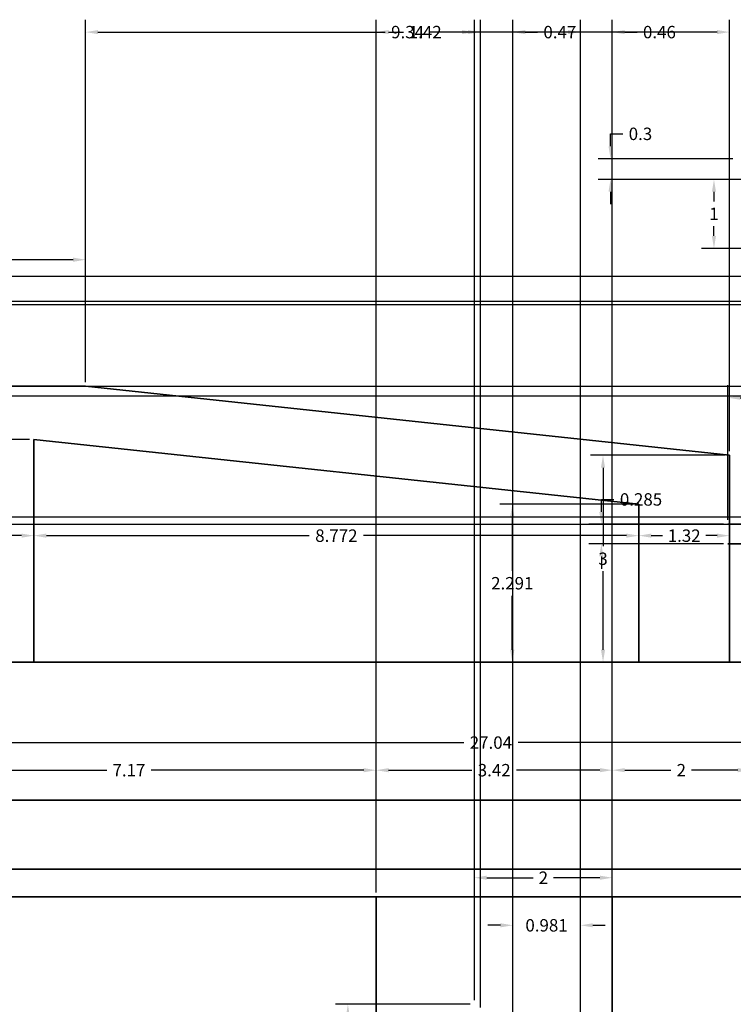
# Model space of a CAD drawing. Units: millimetres. Extents: x 2473 to 2512.3, y 2191.3 to 2230.4.
# Tile 5 of 8: x 2483.3 to 2493.7, y 2216.1 to 2230.4. Entities that reach past the tile are written whole.
import ezdxf

# ---------------------------------------------------------------- set-up
doc = ezdxf.new("R2010")
doc.units = ezdxf.units.MM
doc.layers.add('A-ANNO-DIMS', color=2, linetype='Continuous', lineweight=18)
doc.layers.add('A-ELEV', color=7, linetype='Continuous', lineweight=35)
doc.styles.get("Standard").update_dxf_attribs({"font": 'arial.ttf'})
doc.dimstyles.get("Standard").update_dxf_attribs({"dimtxt": 0.18, "dimasz": 0.18, "dimexe": 0.18, "dimexo": 0.0625, "dimgap": 0.09, "dimtad": 0, "dimtih": 1, "dimtoh": 1, "dimdec": 4, "dimzin": 0, "dimdsep": 46, "dimtxsty": 'Standard', "dimcen": 0.09, "dimadec": 0, "dimazin": 0, "dimtfac": 1, "dimtdec": 4, "dimtofl": 0, "dimtmove": 0, "dimatfit": 3, "dimfxl": 1, "dimtolj": 1, "dimtzin": 0, "dimarcsym": 0})

# ---------------------------------------------------------------- blocks, each defined once
blk = doc.blocks.new('*D18')
at = {"layer": 'A-ANNO-DIMS', "color": 0, "lineweight": -2, "transparency": 16777216}
for p, q in [((2476.623, 2218.117), (2476.623, 2220.07)), ((2503.664, 2218.117), (2503.664, 2220.07)), ((2476.803, 2219.89), (2489.749, 2219.89)), ((2503.484, 2219.89), (2490.538, 2219.89))]:
    blk.add_line(p, q, dxfattribs=at)
at = {"layer": 'A-ANNO-DIMS', "color": 0, "transparency": 16777216}
for points in [[(2476.803, 2219.92), (2476.803, 2219.86), (2476.623, 2219.89)], [(2503.484, 2219.92), (2503.484, 2219.86), (2503.664, 2219.89)]]:
    blk.add_solid(points, dxfattribs=at)
at = {"layer": 'Defpoints', "color": 0, "transparency": 16777216}
for p in [(2503.664, 2219.89), (2476.623, 2218.055), (2503.664, 2218.055)]:
    blk.add_point(p, dxfattribs=at)
at = {"layer": 'A-ANNO-DIMS', "color": 0, "transparency": 16777216, "insert": (2490.143, 2219.89), "char_height": 0.18, "attachment_point": 5}
blk.add_mtext('\\A1;27.04', dxfattribs=at)
blk = doc.blocks.new('*D48')
at = {"layer": 'A-ANNO-DIMS', "color": 0, "lineweight": -2, "transparency": 16777216}
for p, q in [((2481.31, 2217.717), (2481.31, 2219.67)), ((2488.479, 2217.717), (2488.479, 2219.67)), ((2481.49, 2219.49), (2484.571, 2219.49)), ((2488.299, 2219.49), (2485.217, 2219.49))]:
    blk.add_line(p, q, dxfattribs=at)
at = {"layer": 'A-ANNO-DIMS', "color": 0, "transparency": 16777216}
for points in [[(2481.49, 2219.52), (2481.49, 2219.46), (2481.31, 2219.49)], [(2488.299, 2219.52), (2488.299, 2219.46), (2488.479, 2219.49)]]:
    blk.add_solid(points, dxfattribs=at)
at = {"layer": 'Defpoints', "color": 0, "transparency": 16777216}
for p in [(2488.479, 2219.49), (2481.31, 2217.655), (2488.479, 2217.655)]:
    blk.add_point(p, dxfattribs=at)
at = {"layer": 'A-ANNO-DIMS', "color": 0, "transparency": 16777216, "insert": (2484.894, 2219.49), "char_height": 0.18, "attachment_point": 5}
blk.add_mtext('\\A1;7.17', dxfattribs=at)
blk = doc.blocks.new('*D49')
at = {"layer": 'A-ANNO-DIMS', "color": 0, "lineweight": -2, "transparency": 16777216}
for p, q in [((2488.479, 2217.717), (2488.479, 2219.67)), ((2491.904, 2217.717), (2491.904, 2219.67)), ((2488.659, 2219.49), (2489.868, 2219.49)), ((2491.724, 2219.49), (2490.514, 2219.49))]:
    blk.add_line(p, q, dxfattribs=at)
at = {"layer": 'A-ANNO-DIMS', "color": 0, "transparency": 16777216}
for points in [[(2488.659, 2219.52), (2488.659, 2219.46), (2488.479, 2219.49)], [(2491.724, 2219.52), (2491.724, 2219.46), (2491.904, 2219.49)]]:
    blk.add_solid(points, dxfattribs=at)
at = {"layer": 'Defpoints', "color": 0, "transparency": 16777216}
for p in [(2491.904, 2219.49), (2488.479, 2217.655), (2491.904, 2217.655)]:
    blk.add_point(p, dxfattribs=at)
at = {"layer": 'A-ANNO-DIMS', "color": 0, "transparency": 16777216, "insert": (2490.191, 2219.49), "char_height": 0.18, "attachment_point": 5}
blk.add_mtext('\\A1;3.42', dxfattribs=at)
blk = doc.blocks.new('*D50')
at = {"layer": 'A-ANNO-DIMS', "color": 0, "lineweight": -2, "transparency": 16777216}
for p, q in [((2491.904, 2217.717), (2491.904, 2219.67)), ((2493.904, 2217.717), (2493.904, 2219.67)), ((2492.084, 2219.49), (2492.754, 2219.49)), ((2493.724, 2219.49), (2493.053, 2219.49))]:
    blk.add_line(p, q, dxfattribs=at)
at = {"layer": 'A-ANNO-DIMS', "color": 0, "transparency": 16777216}
for points in [[(2492.084, 2219.52), (2492.084, 2219.46), (2491.904, 2219.49)], [(2493.724, 2219.52), (2493.724, 2219.46), (2493.904, 2219.49)]]:
    blk.add_solid(points, dxfattribs=at)
at = {"layer": 'Defpoints', "color": 0, "transparency": 16777216}
for p in [(2493.904, 2219.49), (2491.904, 2217.655), (2493.904, 2217.655)]:
    blk.add_point(p, dxfattribs=at)
at = {"layer": 'A-ANNO-DIMS', "color": 0, "transparency": 16777216, "insert": (2492.904, 2219.49), "char_height": 0.18, "attachment_point": 5}
blk.add_mtext('\\A1;2', dxfattribs=at)
blk = doc.blocks.new('*D56')
at = {"layer": 'A-ANNO-DIMS', "color": 0, "lineweight": -2, "transparency": 16777216}
for p, q in [((2488.479, 2217.717), (2488.479, 2230.37)), ((2489.904, 2216.158), (2489.904, 2230.37)), ((2488.659, 2230.19), (2488.877, 2230.19)), ((2489.724, 2230.19), (2489.506, 2230.19))]:
    blk.add_line(p, q, dxfattribs=at)
at = {"layer": 'A-ANNO-DIMS', "color": 0, "transparency": 16777216}
for points in [[(2488.659, 2230.22), (2488.659, 2230.16), (2488.479, 2230.19)], [(2489.724, 2230.22), (2489.724, 2230.16), (2489.904, 2230.19)]]:
    blk.add_solid(points, dxfattribs=at)
at = {"layer": 'Defpoints', "color": 0, "transparency": 16777216}
for p in [(2489.904, 2230.19), (2488.479, 2217.655), (2489.904, 2216.096)]:
    blk.add_point(p, dxfattribs=at)
at = {"layer": 'A-ANNO-DIMS', "color": 0, "transparency": 16777216, "insert": (2489.191, 2230.19), "char_height": 0.18, "attachment_point": 5}
blk.add_mtext('\\A1;1.42', dxfattribs=at)
blk = doc.blocks.new('*D57')
at = {"layer": 'A-ANNO-DIMS', "color": 0, "lineweight": -2, "transparency": 16777216}
for p, q in [((2489.904, 2216.158), (2489.904, 2218.111)), ((2491.904, 2216.158), (2491.904, 2218.111)), ((2490.084, 2217.931), (2490.754, 2217.931)), ((2491.724, 2217.931), (2491.053, 2217.931))]:
    blk.add_line(p, q, dxfattribs=at)
at = {"layer": 'A-ANNO-DIMS', "color": 0, "transparency": 16777216}
for points in [[(2490.084, 2217.961), (2490.084, 2217.901), (2489.904, 2217.931)], [(2491.724, 2217.961), (2491.724, 2217.901), (2491.904, 2217.931)]]:
    blk.add_solid(points, dxfattribs=at)
at = {"layer": 'Defpoints', "color": 0, "transparency": 16777216}
for p in [(2491.904, 2217.931), (2489.904, 2216.096), (2491.904, 2216.096)]:
    blk.add_point(p, dxfattribs=at)
at = {"layer": 'A-ANNO-DIMS', "color": 0, "transparency": 16777216, "insert": (2490.904, 2217.931), "char_height": 0.18, "attachment_point": 5}
blk.add_mtext('\\A1;2', dxfattribs=at)
blk = doc.blocks.new('*D58')
at = {"layer": 'A-ANNO-DIMS', "color": 0, "lineweight": -2, "transparency": 16777216}
for p, q in [((2490.46, 2215.468), (2490.46, 2217.421)), ((2491.441, 2215.468), (2491.441, 2217.421)), ((2490.28, 2217.241), (2490.1, 2217.241)), ((2491.621, 2217.241), (2491.801, 2217.241))]:
    blk.add_line(p, q, dxfattribs=at)
at = {"layer": 'A-ANNO-DIMS', "color": 0, "transparency": 16777216}
for points in [[(2490.28, 2217.271), (2490.28, 2217.211), (2490.46, 2217.241)], [(2491.621, 2217.271), (2491.621, 2217.211), (2491.441, 2217.241)]]:
    blk.add_solid(points, dxfattribs=at)
at = {"layer": 'Defpoints', "color": 0, "transparency": 16777216}
for p in [(2491.441, 2217.241), (2490.46, 2215.406), (2491.441, 2215.406)]:
    blk.add_point(p, dxfattribs=at)
at = {"layer": 'A-ANNO-DIMS', "color": 0, "transparency": 16777216, "insert": (2490.95, 2217.241), "char_height": 0.18, "attachment_point": 5}
blk.add_mtext('\\A1;0.981', dxfattribs=at)
blk = doc.blocks.new('*D59')
at = {"layer": 'A-ANNO-DIMS', "color": 0, "lineweight": -2, "transparency": 16777216}
for p, q in [((2489.841, 2216.096), (2487.889, 2216.096)), ((2488.069, 2215.916), (2488.069, 2212.957)), ((2488.069, 2209.635), (2488.069, 2212.593)), ((2489.841, 2209.455), (2487.889, 2209.455))]:
    blk.add_line(p, q, dxfattribs=at)
at = {"layer": 'A-ANNO-DIMS', "color": 0, "transparency": 16777216}
for points in [[(2488.039, 2215.916), (2488.099, 2215.916), (2488.069, 2216.096)], [(2488.039, 2209.635), (2488.099, 2209.635), (2488.069, 2209.455)]]:
    blk.add_solid(points, dxfattribs=at)
at = {"layer": 'Defpoints', "color": 0, "transparency": 16777216}
for p in [(2488.069, 2216.096), (2489.904, 2216.096), (2489.904, 2209.455)]:
    blk.add_point(p, dxfattribs=at)
at = {"layer": 'A-ANNO-DIMS', "color": 0, "transparency": 16777216, "insert": (2488.069, 2212.775), "char_height": 0.18, "attachment_point": 5}
blk.add_mtext('\\A1;6.641', dxfattribs=at)
blk = doc.blocks.new('*D72')
at = {"layer": 'A-ANNO-DIMS', "color": 0, "lineweight": -2, "transparency": 16777216}
for p, q in [((2475.623, 2225.117), (2475.623, 2227.07)), ((2484.265, 2225.117), (2484.265, 2227.07)), ((2475.803, 2226.89), (2479.551, 2226.89)), ((2484.085, 2226.89), (2480.337, 2226.89))]:
    blk.add_line(p, q, dxfattribs=at)
at = {"layer": 'A-ANNO-DIMS', "color": 0, "transparency": 16777216}
for points in [[(2475.803, 2226.92), (2475.803, 2226.86), (2475.623, 2226.89)], [(2484.085, 2226.92), (2484.085, 2226.86), (2484.265, 2226.89)]]:
    blk.add_solid(points, dxfattribs=at)
at = {"layer": 'Defpoints', "color": 0, "transparency": 16777216}
for p in [(2484.265, 2226.89), (2475.623, 2225.055), (2484.265, 2225.055)]:
    blk.add_point(p, dxfattribs=at)
at = {"layer": 'A-ANNO-DIMS', "color": 0, "transparency": 16777216, "insert": (2479.944, 2226.89), "char_height": 0.18, "attachment_point": 5}
blk.add_mtext('\\A1;8.642', dxfattribs=at)
blk = doc.blocks.new('*D73')
at = {"layer": 'A-ANNO-DIMS', "color": 0, "lineweight": -2, "transparency": 16777216}
for p, q in [((2484.265, 2225.117), (2484.265, 2230.37)), ((2493.604, 2224.117), (2493.604, 2230.37)), ((2484.445, 2230.19), (2488.611, 2230.19)), ((2493.424, 2230.19), (2489.258, 2230.19))]:
    blk.add_line(p, q, dxfattribs=at)
at = {"layer": 'A-ANNO-DIMS', "color": 0, "transparency": 16777216}
for points in [[(2484.445, 2230.22), (2484.445, 2230.16), (2484.265, 2230.19)], [(2493.424, 2230.22), (2493.424, 2230.16), (2493.604, 2230.19)]]:
    blk.add_solid(points, dxfattribs=at)
at = {"layer": 'Defpoints', "color": 0, "transparency": 16777216}
for p in [(2493.604, 2230.19), (2484.265, 2225.055), (2493.604, 2224.055)]:
    blk.add_point(p, dxfattribs=at)
at = {"layer": 'A-ANNO-DIMS', "color": 0, "transparency": 16777216, "insert": (2488.935, 2230.19), "char_height": 0.18, "attachment_point": 5}
blk.add_mtext('\\A1;9.34', dxfattribs=at)
blk = doc.blocks.new('*D74')
at = {"layer": 'A-ANNO-DIMS', "color": 0, "lineweight": -2, "transparency": 16777216}
for p, q in [((2493.542, 2224.055), (2491.589, 2224.055)), ((2491.769, 2223.875), (2491.769, 2222.737)), ((2491.769, 2221.235), (2491.769, 2222.373)), ((2493.542, 2221.055), (2491.589, 2221.055))]:
    blk.add_line(p, q, dxfattribs=at)
at = {"layer": 'A-ANNO-DIMS', "color": 0, "transparency": 16777216}
for points in [[(2491.739, 2223.875), (2491.799, 2223.875), (2491.769, 2224.055)], [(2491.739, 2221.235), (2491.799, 2221.235), (2491.769, 2221.055)]]:
    blk.add_solid(points, dxfattribs=at)
at = {"layer": 'Defpoints', "color": 0, "transparency": 16777216}
for p in [(2491.769, 2224.055), (2493.604, 2224.055), (2493.604, 2221.055)]:
    blk.add_point(p, dxfattribs=at)
at = {"layer": 'A-ANNO-DIMS', "color": 0, "transparency": 16777216, "insert": (2491.769, 2222.555), "char_height": 0.18, "attachment_point": 5}
blk.add_mtext('\\A1;3', dxfattribs=at)
blk = doc.blocks.new('*D75')
at = {"layer": 'A-ANNO-DIMS', "color": 0, "lineweight": -2, "transparency": 16777216}
for p, q in [((2483.453, 2224.285), (2481.501, 2224.285)), ((2481.681, 2224.105), (2481.681, 2222.852)), ((2481.681, 2221.235), (2481.681, 2222.488)), ((2483.453, 2221.055), (2481.501, 2221.055))]:
    blk.add_line(p, q, dxfattribs=at)
at = {"layer": 'A-ANNO-DIMS', "color": 0, "transparency": 16777216}
for points in [[(2481.651, 2224.105), (2481.711, 2224.105), (2481.681, 2224.285)], [(2481.651, 2221.235), (2481.711, 2221.235), (2481.681, 2221.055)]]:
    blk.add_solid(points, dxfattribs=at)
at = {"layer": 'Defpoints', "color": 0, "transparency": 16777216}
for p in [(2481.681, 2224.285), (2483.516, 2224.285), (2483.516, 2221.055)]:
    blk.add_point(p, dxfattribs=at)
at = {"layer": 'A-ANNO-DIMS', "color": 0, "transparency": 16777216, "insert": (2481.681, 2222.67), "char_height": 0.18, "attachment_point": 5}
blk.add_mtext('\\A1;3.23', dxfattribs=at)
blk = doc.blocks.new('*D76')
at = {"layer": 'A-ANNO-DIMS', "color": 0, "lineweight": -2, "transparency": 16777216}
for p, q in [((2492.225, 2223.346), (2490.273, 2223.346)), ((2490.453, 2223.166), (2490.453, 2222.382)), ((2490.453, 2221.235), (2490.453, 2222.018)), ((2492.225, 2221.055), (2490.273, 2221.055))]:
    blk.add_line(p, q, dxfattribs=at)
at = {"layer": 'A-ANNO-DIMS', "color": 0, "transparency": 16777216}
for points in [[(2490.423, 2223.166), (2490.483, 2223.166), (2490.453, 2223.346)], [(2490.423, 2221.235), (2490.483, 2221.235), (2490.453, 2221.055)]]:
    blk.add_solid(points, dxfattribs=at)
at = {"layer": 'Defpoints', "color": 0, "transparency": 16777216}
for p in [(2490.453, 2223.346), (2492.288, 2223.346), (2492.288, 2221.055)]:
    blk.add_point(p, dxfattribs=at)
at = {"layer": 'A-ANNO-DIMS', "color": 0, "transparency": 16777216, "insert": (2490.453, 2222.2), "char_height": 0.18, "attachment_point": 5}
blk.add_mtext('\\A1;2.291', dxfattribs=at)
blk = doc.blocks.new('*D77')
at = {"layer": 'A-ANNO-DIMS', "color": 0, "lineweight": -2, "transparency": 16777216}
for p, q in [((2475.623, 2221.117), (2475.623, 2223.07)), ((2483.516, 2221.117), (2483.516, 2223.07)), ((2475.803, 2222.89), (2479.176, 2222.89)), ((2483.336, 2222.89), (2479.962, 2222.89))]:
    blk.add_line(p, q, dxfattribs=at)
at = {"layer": 'A-ANNO-DIMS', "color": 0, "transparency": 16777216}
for points in [[(2475.803, 2222.92), (2475.803, 2222.86), (2475.623, 2222.89)], [(2483.336, 2222.92), (2483.336, 2222.86), (2483.516, 2222.89)]]:
    blk.add_solid(points, dxfattribs=at)
at = {"layer": 'Defpoints', "color": 0, "transparency": 16777216}
for p in [(2483.516, 2222.89), (2475.623, 2221.055), (2483.516, 2221.055)]:
    blk.add_point(p, dxfattribs=at)
at = {"layer": 'A-ANNO-DIMS', "color": 0, "transparency": 16777216, "insert": (2479.569, 2222.89), "char_height": 0.18, "attachment_point": 5}
blk.add_mtext('\\A1;7.893', dxfattribs=at)
blk = doc.blocks.new('*D78')
at = {"layer": 'A-ANNO-DIMS', "color": 0, "lineweight": -2, "transparency": 16777216}
for p, q in [((2483.516, 2221.117), (2483.516, 2223.07)), ((2492.288, 2221.117), (2492.288, 2223.07)), ((2483.696, 2222.89), (2487.509, 2222.89)), ((2492.108, 2222.89), (2488.295, 2222.89))]:
    blk.add_line(p, q, dxfattribs=at)
at = {"layer": 'A-ANNO-DIMS', "color": 0, "transparency": 16777216}
for points in [[(2483.696, 2222.92), (2483.696, 2222.86), (2483.516, 2222.89)], [(2492.108, 2222.92), (2492.108, 2222.86), (2492.288, 2222.89)]]:
    blk.add_solid(points, dxfattribs=at)
at = {"layer": 'Defpoints', "color": 0, "transparency": 16777216}
for p in [(2492.288, 2222.89), (2483.516, 2221.055), (2492.288, 2221.055)]:
    blk.add_point(p, dxfattribs=at)
at = {"layer": 'A-ANNO-DIMS', "color": 0, "transparency": 16777216, "insert": (2487.902, 2222.89), "char_height": 0.18, "attachment_point": 5}
blk.add_mtext('\\A1;8.772', dxfattribs=at)
blk = doc.blocks.new('*D79')
at = {"layer": 'A-ANNO-DIMS', "color": 0, "lineweight": -2, "transparency": 16777216}
for p, q in [((2492.288, 2221.117), (2492.288, 2223.07)), ((2493.604, 2221.117), (2493.604, 2223.07)), ((2492.468, 2222.89), (2492.632, 2222.89)), ((2493.424, 2222.89), (2493.26, 2222.89))]:
    blk.add_line(p, q, dxfattribs=at)
at = {"layer": 'A-ANNO-DIMS', "color": 0, "transparency": 16777216}
for points in [[(2492.468, 2222.92), (2492.468, 2222.86), (2492.288, 2222.89)], [(2493.424, 2222.92), (2493.424, 2222.86), (2493.604, 2222.89)]]:
    blk.add_solid(points, dxfattribs=at)
at = {"layer": 'Defpoints', "color": 0, "transparency": 16777216}
for p in [(2493.604, 2222.89), (2492.288, 2221.055), (2493.604, 2221.055)]:
    blk.add_point(p, dxfattribs=at)
at = {"layer": 'A-ANNO-DIMS', "color": 0, "transparency": 16777216, "insert": (2492.946, 2222.89), "char_height": 0.18, "attachment_point": 5}
blk.add_mtext('\\A1;1.32', dxfattribs=at)
blk = doc.blocks.new('*D80')
at = {"layer": 'A-ANNO-DIMS', "color": 0, "lineweight": -2, "transparency": 16777216}
for p, q in [((2491.745, 2223.235), (2491.745, 2223.415)), ((2491.745, 2223.415), (2491.925, 2223.415)), ((2493.518, 2223.055), (2491.565, 2223.055)), ((2493.518, 2222.77), (2491.565, 2222.77)), ((2491.745, 2222.59), (2491.745, 2222.41))]:
    blk.add_line(p, q, dxfattribs=at)
at = {"layer": 'A-ANNO-DIMS', "color": 0, "transparency": 16777216}
for points in [[(2491.715, 2223.235), (2491.775, 2223.235), (2491.745, 2223.055)], [(2491.715, 2222.59), (2491.775, 2222.59), (2491.745, 2222.77)]]:
    blk.add_solid(points, dxfattribs=at)
at = {"layer": 'Defpoints', "color": 0, "transparency": 16777216}
for p in [(2491.745, 2223.055), (2493.58, 2223.055), (2493.58, 2222.77)]:
    blk.add_point(p, dxfattribs=at)
at = {"layer": 'A-ANNO-DIMS', "color": 0, "transparency": 16777216, "insert": (2492.32, 2223.415), "char_height": 0.18, "attachment_point": 5}
blk.add_mtext('\\A1;0.285', dxfattribs=at)
blk = doc.blocks.new('*D81')
at = {"layer": 'A-ANNO-DIMS', "color": 0, "lineweight": -2, "transparency": 16777216}
for p, q in [((2493.58, 2223.117), (2493.58, 2225.07)), ((2495.803, 2223.117), (2495.803, 2225.07)), ((2493.76, 2224.89), (2494.297, 2224.89)), ((2495.623, 2224.89), (2495.087, 2224.89))]:
    blk.add_line(p, q, dxfattribs=at)
at = {"layer": 'A-ANNO-DIMS', "color": 0, "transparency": 16777216}
for points in [[(2493.76, 2224.92), (2493.76, 2224.86), (2493.58, 2224.89)], [(2495.623, 2224.92), (2495.623, 2224.86), (2495.803, 2224.89)]]:
    blk.add_solid(points, dxfattribs=at)
at = {"layer": 'Defpoints', "color": 0, "transparency": 16777216}
for p in [(2495.803, 2224.89), (2493.58, 2223.055), (2495.803, 2223.055)]:
    blk.add_point(p, dxfattribs=at)
at = {"layer": 'A-ANNO-DIMS', "color": 0, "transparency": 16777216, "insert": (2494.692, 2224.89), "char_height": 0.18, "attachment_point": 5}
blk.add_mtext('\\A1;2.223', dxfattribs=at)
blk = doc.blocks.new('*D85')
at = {"layer": 'A-ANNO-DIMS', "color": 0, "lineweight": -2, "transparency": 16777216}
for p, q in [((2495.15, 2228.055), (2493.198, 2228.055)), ((2493.378, 2227.875), (2493.378, 2227.735)), ((2493.378, 2227.235), (2493.378, 2227.375)), ((2495.15, 2227.055), (2493.198, 2227.055))]:
    blk.add_line(p, q, dxfattribs=at)
at = {"layer": 'A-ANNO-DIMS', "color": 0, "transparency": 16777216}
for points in [[(2493.348, 2227.875), (2493.408, 2227.875), (2493.378, 2228.055)], [(2493.348, 2227.235), (2493.408, 2227.235), (2493.378, 2227.055)]]:
    blk.add_solid(points, dxfattribs=at)
at = {"layer": 'Defpoints', "color": 0, "transparency": 16777216}
for p in [(2493.378, 2228.055), (2495.213, 2228.055), (2495.213, 2227.055)]:
    blk.add_point(p, dxfattribs=at)
at = {"layer": 'A-ANNO-DIMS', "color": 0, "transparency": 16777216, "insert": (2493.378, 2227.555), "char_height": 0.18, "attachment_point": 5}
blk.add_mtext('\\A1;1', dxfattribs=at)
blk = doc.blocks.new('*D86')
at = {"layer": 'A-ANNO-DIMS', "color": 0, "lineweight": -2, "transparency": 16777216}
for p, q in [((2491.878, 2228.535), (2491.878, 2228.715)), ((2491.878, 2228.715), (2492.058, 2228.715)), ((2493.65, 2228.355), (2491.698, 2228.355)), ((2493.65, 2228.055), (2491.698, 2228.055)), ((2491.878, 2227.875), (2491.878, 2227.695))]:
    blk.add_line(p, q, dxfattribs=at)
at = {"layer": 'A-ANNO-DIMS', "color": 0, "transparency": 16777216}
for points in [[(2491.848, 2228.535), (2491.908, 2228.535), (2491.878, 2228.355)], [(2491.848, 2227.875), (2491.908, 2227.875), (2491.878, 2228.055)]]:
    blk.add_solid(points, dxfattribs=at)
at = {"layer": 'Defpoints', "color": 0, "transparency": 16777216}
for p in [(2491.878, 2228.355), (2493.713, 2228.355), (2493.713, 2228.055)]:
    blk.add_point(p, dxfattribs=at)
at = {"layer": 'A-ANNO-DIMS', "color": 0, "transparency": 16777216, "insert": (2492.312, 2228.715), "char_height": 0.18, "attachment_point": 5}
blk.add_mtext('\\A1;0.3', dxfattribs=at)
blk = doc.blocks.new('*D100')
at = {"layer": 'A-ANNO-DIMS', "color": 0, "lineweight": -2, "transparency": 16777216}
for p, q in [((2489.991, 2216.05), (2489.991, 2230.37)), ((2490.46, 2215.468), (2490.46, 2230.37)), ((2489.811, 2230.19), (2489.631, 2230.19)), ((2490.64, 2230.19), (2490.82, 2230.19))]:
    blk.add_line(p, q, dxfattribs=at)
at = {"layer": 'A-ANNO-DIMS', "color": 0, "transparency": 16777216}
for points in [[(2489.811, 2230.22), (2489.811, 2230.16), (2489.991, 2230.19)], [(2490.64, 2230.22), (2490.64, 2230.16), (2490.46, 2230.19)]]:
    blk.add_solid(points, dxfattribs=at)
at = {"layer": 'Defpoints', "color": 0, "transparency": 16777216}
for p in [(2490.46, 2230.19), (2489.991, 2215.987), (2490.46, 2215.406)]:
    blk.add_point(p, dxfattribs=at)
at = {"layer": 'A-ANNO-DIMS', "color": 0, "transparency": 16777216, "insert": (2491.143, 2230.19), "char_height": 0.18, "attachment_point": 5}
blk.add_mtext('\\A1;0.47', dxfattribs=at)
blk = doc.blocks.new('*D101')
at = {"layer": 'A-ANNO-DIMS', "color": 0, "lineweight": -2, "transparency": 16777216}
for p, q in [((2491.441, 2215.468), (2491.441, 2230.37)), ((2491.904, 2216.05), (2491.904, 2230.37)), ((2491.261, 2230.19), (2491.081, 2230.19)), ((2492.084, 2230.19), (2492.264, 2230.19))]:
    blk.add_line(p, q, dxfattribs=at)
at = {"layer": 'A-ANNO-DIMS', "color": 0, "transparency": 16777216}
for points in [[(2491.261, 2230.22), (2491.261, 2230.16), (2491.441, 2230.19)], [(2492.084, 2230.22), (2492.084, 2230.16), (2491.904, 2230.19)]]:
    blk.add_solid(points, dxfattribs=at)
at = {"layer": 'Defpoints', "color": 0, "transparency": 16777216}
for p in [(2491.904, 2230.19), (2491.904, 2215.987), (2491.441, 2215.406)]:
    blk.add_point(p, dxfattribs=at)
at = {"layer": 'A-ANNO-DIMS', "color": 0, "transparency": 16777216, "insert": (2492.587, 2230.19), "char_height": 0.18, "attachment_point": 5}
blk.add_mtext('\\A1;0.46', dxfattribs=at)
blk = doc.blocks.new('*D123')
at = {"layer": 'A-ANNO-DIMS', "color": 0, "lineweight": -2, "transparency": 16777216}
for p, q in [((2473.788, 2226.825), (2473.788, 2227.005)), ((2498.65, 2226.645), (2473.608, 2226.645)), ((2498.79, 2226.285), (2473.608, 2226.285)), ((2473.788, 2226.105), (2473.788, 2225.925)), ((2473.788, 2225.925), (2473.608, 2225.925))]:
    blk.add_line(p, q, dxfattribs=at)
at = {"layer": 'A-ANNO-DIMS', "color": 0, "transparency": 16777216}
for points in [[(2473.758, 2226.825), (2473.818, 2226.825), (2473.788, 2226.645)], [(2473.758, 2226.105), (2473.818, 2226.105), (2473.788, 2226.285)]]:
    blk.add_solid(points, dxfattribs=at)
at = {"layer": 'Defpoints', "color": 0, "transparency": 16777216}
for p in [(2498.713, 2226.645), (2473.788, 2226.285), (2498.852, 2226.285)]:
    blk.add_point(p, dxfattribs=at)
at = {"layer": 'A-ANNO-DIMS', "color": 0, "transparency": 16777216, "insert": (2473.284, 2225.925), "char_height": 0.18, "attachment_point": 5}
blk.add_mtext('\\A1;0.36', dxfattribs=at)
blk = doc.blocks.new('*D124')
at = {"layer": 'A-ANNO-DIMS', "color": 0, "lineweight": -2, "transparency": 16777216}
for p, q in [((2473.788, 2226.465), (2473.788, 2226.645)), ((2498.79, 2226.285), (2473.608, 2226.285)), ((2498.832, 2226.235), (2473.608, 2226.235)), ((2473.788, 2226.055), (2473.788, 2225.875)), ((2473.788, 2225.875), (2473.608, 2225.875))]:
    blk.add_line(p, q, dxfattribs=at)
at = {"layer": 'A-ANNO-DIMS', "color": 0, "transparency": 16777216}
for points in [[(2473.758, 2226.465), (2473.818, 2226.465), (2473.788, 2226.285)], [(2473.758, 2226.055), (2473.818, 2226.055), (2473.788, 2226.235)]]:
    blk.add_solid(points, dxfattribs=at)
at = {"layer": 'Defpoints', "color": 0, "transparency": 16777216}
for p in [(2473.788, 2226.235), (2498.852, 2226.285), (2498.894, 2226.235)]:
    blk.add_point(p, dxfattribs=at)
at = {"layer": 'A-ANNO-DIMS', "color": 0, "transparency": 16777216, "insert": (2473.283, 2225.875), "char_height": 0.18, "attachment_point": 5}
blk.add_mtext('\\A1;0.05', dxfattribs=at)
blk = doc.blocks.new('*D130')
at = {"layer": 'A-ANNO-DIMS', "color": 0, "lineweight": -2, "transparency": 16777216}
for p, q in [((2511.548, 2225.235), (2511.548, 2225.415)), ((2481.978, 2225.055), (2511.728, 2225.055)), ((2481.869, 2224.915), (2511.728, 2224.915)), ((2511.548, 2224.735), (2511.548, 2224.555)), ((2511.548, 2224.555), (2511.368, 2224.555))]:
    blk.add_line(p, q, dxfattribs=at)
at = {"layer": 'A-ANNO-DIMS', "color": 0, "transparency": 16777216}
for points in [[(2511.518, 2225.235), (2511.578, 2225.235), (2511.548, 2225.055)], [(2511.518, 2224.735), (2511.578, 2224.735), (2511.548, 2224.915)]]:
    blk.add_solid(points, dxfattribs=at)
at = {"layer": 'Defpoints', "color": 0, "transparency": 16777216}
for p in [(2481.915, 2225.055), (2481.806, 2224.915), (2511.548, 2224.915)]:
    blk.add_point(p, dxfattribs=at)
at = {"layer": 'A-ANNO-DIMS', "color": 0, "transparency": 16777216, "insert": (2511.044, 2224.555), "char_height": 0.18, "attachment_point": 5}
blk.add_mtext('\\A1;0.14', dxfattribs=at)
blk = doc.blocks.new('*D131')
at = {"layer": 'A-ANNO-DIMS', "color": 0, "lineweight": -2, "transparency": 16777216}
for p, q in [((2511.548, 2223.343), (2511.548, 2223.523)), ((2511.548, 2223.523), (2511.728, 2223.523)), ((2481.869, 2223.163), (2511.728, 2223.163)), ((2481.978, 2223.055), (2511.728, 2223.055)), ((2511.548, 2222.875), (2511.548, 2222.695))]:
    blk.add_line(p, q, dxfattribs=at)
at = {"layer": 'A-ANNO-DIMS', "color": 0, "transparency": 16777216}
for points in [[(2511.518, 2223.343), (2511.578, 2223.343), (2511.548, 2223.163)], [(2511.518, 2222.875), (2511.578, 2222.875), (2511.548, 2223.055)]]:
    blk.add_solid(points, dxfattribs=at)
at = {"layer": 'Defpoints', "color": 0, "transparency": 16777216}
for p in [(2481.806, 2223.163), (2481.915, 2223.055), (2511.548, 2223.163)]:
    blk.add_point(p, dxfattribs=at)
at = {"layer": 'A-ANNO-DIMS', "color": 0, "transparency": 16777216, "insert": (2512.034, 2223.523), "char_height": 0.18, "attachment_point": 5}
blk.add_mtext('\\A1;0.11', dxfattribs=at)

msp = doc.modelspace()

# ---------------------------------------------------------------- linework, layer by layer
at = {"layer": 'A-ELEV'}
for p, q in [((2475.6229, 2225.0549), (2484.2649, 2225.0549)), ((2484.2649, 2225.0549), (2493.6042, 2224.0549)), ((2492.2878, 2223.3457), (2483.5156, 2224.285)), ((2483.5156, 2224.285), (2483.5156, 2221.0549)), ((2493.6042, 2221.0549), (2493.6042, 2224.0549)), ((2492.2878, 2221.0549), (2492.2878, 2223.3457)), ((2495.8034, 2223.0549), (2493.5802, 2223.0549)), ((2506.7629, 2222.7699), (2493.5802, 2222.7699)), ((2506.7629, 2221.0549), (2475.6229, 2221.0549)), ((2506.7629, 2219.0549), (2475.6229, 2219.0549)), ((2503.6639, 2218.0549), (2476.6229, 2218.0549)), ((2477.0229, 2217.6549), (2503.0616, 2217.6549)), ((2488.4789, 2209.4549), (2488.4789, 2217.6549)), ((2491.9035, 2217.6549), (2491.9035, 2207.4549))]:
    msp.add_line(p, q, dxfattribs=at)

# ---------------------------------------------------------------- dimensions: what is measured, and where the dimension line sits
at = {"layer": 'A-ANNO-DIMS'}
for base, p1, p2, override, picture, middle in [((2493.6042, 2230.1899), (2484.2649, 2225.0549), (2493.6042, 2224.0549), {"dimdec": 2, "dimlfac": 1, "dimrnd": 0, "dimzin": 0, "dimdsep": 46, "dimlunit": 2}, '*D73', (2488.9345, 2230.1899)), ((2489.9035, 2230.1899), (2488.4789, 2217.6549), (2489.9035, 2216.0958), {"dimdec": 2, "dimlfac": 1, "dimrnd": 0, "dimzin": 0, "dimdsep": 46, "dimlunit": 2}, '*D56', (2489.1912, 2230.1899)), ((2490.4596, 2230.1899), (2489.9911, 2215.9871), (2490.4596, 2215.406), {"dimdec": 2, "dimlfac": 1, "dimrnd": 0, "dimzin": 0, "dimdsep": 46, "dimlunit": 2}, '*D100', (2491.1434, 2230.1899)), ((2491.9035, 2230.1899), (2491.4406, 2215.406), (2491.9035, 2215.9871), {"dimdec": 2, "dimlfac": 1, "dimrnd": 0, "dimzin": 0, "dimdsep": 46, "dimlunit": 2}, '*D101', (2492.5872, 2230.1899)), ((2484.2649, 2226.8899), (2475.6229, 2225.0549), (2484.2649, 2225.0549), {"dimdec": 3, "dimlfac": 1, "dimrnd": 0, "dimzin": 0, "dimdsep": 46, "dimlunit": 2}, '*D72', (2479.9439, 2226.8899)), ((2495.8034, 2224.8899), (2493.5802, 2223.0549), (2495.8034, 2223.0549), {"dimdec": 3, "dimlfac": 1, "dimrnd": 0, "dimzin": 0, "dimdsep": 46, "dimlunit": 2}, '*D81', (2494.6918, 2224.8899)), ((2483.5156, 2222.8899), (2475.6229, 2221.0549), (2483.5156, 2221.0549), {"dimdec": 3, "dimlfac": 1, "dimrnd": 0, "dimzin": 0, "dimdsep": 46, "dimlunit": 2}, '*D77', (2479.5693, 2222.8899)), ((2492.2878, 2222.8899), (2483.5156, 2221.0549), (2492.2878, 2221.0549), {"dimdec": 3, "dimlfac": 1, "dimrnd": 0, "dimzin": 0, "dimdsep": 46, "dimlunit": 2}, '*D78', (2487.9017, 2222.8899)), ((2493.6042, 2222.8899), (2492.2878, 2221.0549), (2493.6042, 2221.0549), {"dimdec": 2, "dimlfac": 1, "dimrnd": 0, "dimzin": 0, "dimdsep": 46, "dimlunit": 2}, '*D79', (2492.946, 2222.8899)), ((2503.6639, 2219.8899), (2476.6229, 2218.0549), (2503.6639, 2218.0549), {"dimdec": 2, "dimlfac": 1, "dimrnd": 0, "dimzin": 0, "dimdsep": 46, "dimlunit": 2}, '*D18', (2490.1434, 2219.8899)), ((2488.4789, 2219.4899), (2481.3096, 2217.6549), (2488.4789, 2217.6549), {"dimdec": 2, "dimlfac": 1, "dimrnd": 0, "dimzin": 0, "dimdsep": 46, "dimlunit": 2}, '*D48', (2484.8943, 2219.4899)), ((2491.9035, 2219.4899), (2488.4789, 2217.6549), (2491.9035, 2217.6549), {"dimdec": 2, "dimlfac": 1, "dimrnd": 0, "dimzin": 0, "dimdsep": 46, "dimlunit": 2}, '*D49', (2490.1912, 2219.4899)), ((2493.9035, 2219.4899), (2491.9035, 2217.6549), (2493.9035, 2217.6549), {"dimdec": 0, "dimlfac": 1, "dimrnd": 0, "dimzin": 0, "dimdsep": 46, "dimlunit": 2}, '*D50', (2492.9035, 2219.4899)), ((2491.9035, 2217.9308), (2489.9035, 2216.0958), (2491.9035, 2216.0958), {"dimdec": 0, "dimlfac": 1, "dimrnd": 0, "dimzin": 0, "dimdsep": 46, "dimlunit": 2}, '*D57', (2490.9035, 2217.9308)), ((2491.4406, 2217.241), (2490.4596, 2215.406), (2491.4406, 2215.406), {"dimdec": 3, "dimlfac": 1, "dimrnd": 0, "dimzin": 0, "dimdsep": 46, "dimlunit": 2}, '*D58', (2490.9501, 2217.241))]:
    dim = msp.add_linear_dim(base=base, p1=p1, p2=p2, dimstyle='Standard', override=override, dxfattribs=at)
    dim.commit()
    dim.dimension.update_dxf_attribs({"geometry": picture, "text_midpoint": middle})
for base, p1, p2, override, picture, middle in [((2491.8779, 2228.3549), (2493.7129, 2228.0549), (2493.7129, 2228.3549), {"dimdec": 1, "dimlfac": 1, "dimrnd": 0, "dimzin": 0, "dimdsep": 46, "dimlunit": 2}, '*D86', (2492.3118, 2228.7149)), ((2493.3779, 2228.0549), (2495.2129, 2227.0549), (2495.2129, 2228.0549), {"dimdec": 0, "dimlfac": 1, "dimrnd": 0, "dimzin": 0, "dimdsep": 46, "dimlunit": 2}, '*D85', (2493.3779, 2227.5549)), ((2473.7879, 2226.2854), (2498.7129, 2226.6451), (2498.8524, 2226.2854), {"dimdec": 2, "dimlfac": 1, "dimrnd": 0, "dimzin": 0, "dimdsep": 46, "dimlunit": 2}, '*D123', (2473.2842, 2225.9254)), ((2473.7879, 2226.2352), (2498.8524, 2226.2854), (2498.8944, 2226.2352), {"dimdec": 2, "dimlfac": 1, "dimrnd": 0, "dimzin": 0, "dimdsep": 46, "dimlunit": 2}, '*D124', (2473.2834, 2225.8752)), ((2511.5479, 2224.9147), (2481.9154, 2225.0549), (2481.806, 2224.9147), {"dimdec": 2, "dimlfac": 1, "dimrnd": 0, "dimzin": 0, "dimdsep": 46, "dimlunit": 2}, '*D130', (2511.0445, 2224.5547)), ((2481.6806, 2224.285), (2483.5156, 2221.0549), (2483.5156, 2224.285), {"dimdec": 2, "dimlfac": 1, "dimrnd": 0, "dimzin": 0, "dimdsep": 46, "dimlunit": 2}, '*D75', (2481.6806, 2222.6699)), ((2491.7692, 2224.0549), (2493.6042, 2221.0549), (2493.6042, 2224.0549), {"dimdec": 0, "dimlfac": 1, "dimrnd": 0, "dimzin": 0, "dimdsep": 46, "dimlunit": 2}, '*D74', (2491.7692, 2222.5549)), ((2511.5479, 2223.1632), (2481.9154, 2223.0549), (2481.806, 2223.1632), {"dimdec": 2, "dimlfac": 1, "dimrnd": 0, "dimzin": 0, "dimdsep": 46, "dimlunit": 2}, '*D131', (2512.0343, 2223.5232)), ((2491.7452, 2223.0549), (2493.5802, 2222.7699), (2493.5802, 2223.0549), {"dimdec": 3, "dimlfac": 1, "dimrnd": 0, "dimzin": 0, "dimdsep": 46, "dimlunit": 2}, '*D80', (2492.3196, 2223.4149)), ((2490.4528, 2223.3457), (2492.2878, 2221.0549), (2492.2878, 2223.3457), {"dimdec": 3, "dimlfac": 1, "dimrnd": 0, "dimzin": 0, "dimdsep": 46, "dimlunit": 2}, '*D76', (2490.4528, 2222.2003)), ((2488.0685, 2216.0958), (2489.9035, 2209.4549), (2489.9035, 2216.0958), {"dimdec": 3, "dimlfac": 1, "dimrnd": 0, "dimzin": 0, "dimdsep": 46, "dimlunit": 2}, '*D59', (2488.0685, 2212.7753))]:
    dim = msp.add_linear_dim(base=base, p1=p1, p2=p2, angle=90, dimstyle='Standard', override=override, dxfattribs=at)
    dim.commit()
    dim.dimension.update_dxf_attribs({"geometry": picture, "text_midpoint": middle})

doc.saveas('drawing.dxf')
